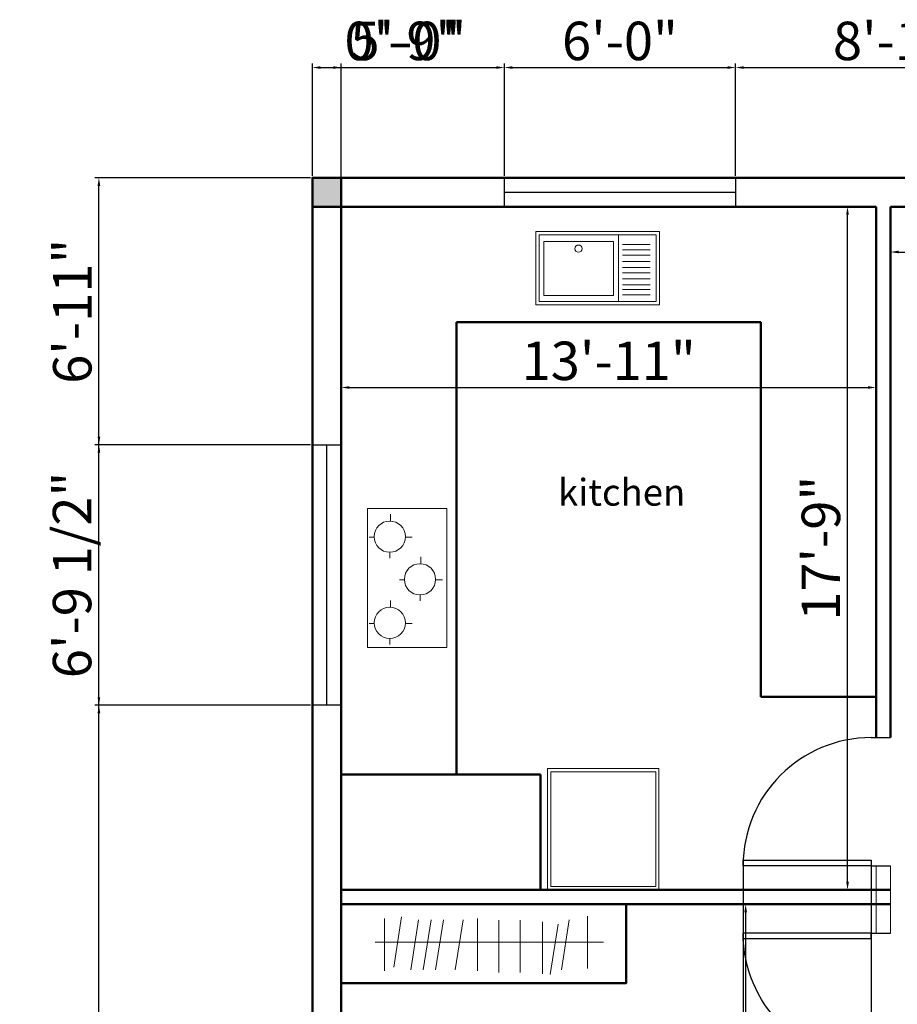
# Model space of a CAD drawing. Units: inches. Extents: x 1367 to 2309, y 1406 to 3826.
# Tile 2 of 9: x 1417 to 1691, y 1853 to 2160. Entities that reach past the tile are written whole.
import ezdxf

# ---------------------------------------------------------------- set-up
doc = ezdxf.new("R2010")
doc.units = ezdxf.units.IN
for name, color, linetype, lineweight in [('A-ANNO-DIMS', 2, 'Continuous', 18), ('A-AREA-IDEN', 3, 'Continuous', 18), ('A-DOOR', 4, 'Continuous', 25), ('A-FLOR-FIXT', 8, 'Continuous', 18), ('A-FURN', 8, 'Continuous', 18), ('A-GLAZ', 4, 'Continuous', 25), ('A-WALL', 7, 'Continuous', 50), ('A-WALL-PATT', 8, 'Continuous', 18)]:
    doc.layers.add(name, color=color, linetype=linetype, lineweight=lineweight)
doc.styles.get("Standard").update_dxf_attribs({"font": 'arial.ttf'})
doc.dimstyles.new('ISO-25', dxfattribs={"dimtxt": 12, "dimasz": 2.5, "dimexe": 1.25, "dimexo": 0.625, "dimtad": 1, "dimdec": 0, "dimlunit": 4, "dimtxsty": 'Standard', "dimcen": 2.5, "dimadec": 0, "dimazin": 0, "dimtfac": 1, "dimtdec": 0, "dimtmove": 0, "dimatfit": 3, "dimfxl": 1, "dimarcsym": 0})

# ---------------------------------------------------------------- blocks, each defined once
blk = doc.blocks.new('*U2')
for p, q in [((0, 0), (0, -6)), ((40, 0), (40, -6))]:
    blk.add_line(p, q)
blk.add_lwpolyline([(0, 0), (0, 40), (1.75, 40), (1.75, 0)], close=True)
blk.add_arc((0, 0), 40, 0, 90)
blk = doc.blocks.new('*D23')
at = {"layer": 'A-ANNO-DIMS', "color": 0, "lineweight": -2, "transparency": 16777216}
for p, q in [((1517.49, 2101.5), (1517.49, 2044.48)), ((1684.37, 2101.5), (1684.37, 2044.48)), ((1519.99, 2045.73), (1681.87, 2045.73))]:
    blk.add_line(p, q, dxfattribs=at)
at = {"layer": 'A-ANNO-DIMS', "color": 0, "lineweight": 100, "transparency": 16777216}
for points in [[(1519.99, 2046.15), (1519.99, 2045.32), (1517.49, 2045.73)], [(1681.87, 2046.15), (1681.87, 2045.32), (1684.37, 2045.73)]]:
    blk.add_solid(points, dxfattribs=at)
at = {"layer": 'Defpoints', "color": 0, "lineweight": 100, "transparency": 16777216}
for p in [(1517.49, 2102.13), (1684.37, 2102.13), (1684.37, 2045.73)]:
    blk.add_point(p, dxfattribs=at)
at = {"layer": 'A-ANNO-DIMS', "color": 0, "transparency": 16777216, "insert": (1600.93, 2052.49), "char_height": 12, "attachment_point": 5}
blk.add_mtext('13\'-11"', dxfattribs=at)
blk = doc.blocks.new('*D24')
at = {"layer": 'A-ANNO-DIMS', "color": 0, "lineweight": -2, "transparency": 16777216}
for p, q in [((1683.74, 2102.13), (1674.21, 2102.13)), ((1675.46, 1891.56), (1675.46, 2099.63)), ((1683.74, 1889.06), (1674.21, 1889.06))]:
    blk.add_line(p, q, dxfattribs=at)
at = {"layer": 'A-ANNO-DIMS', "color": 0, "lineweight": 100, "transparency": 16777216}
for points in [[(1675.04, 2099.63), (1675.88, 2099.63), (1675.46, 2102.13)], [(1675.04, 1891.56), (1675.88, 1891.56), (1675.46, 1889.06)]]:
    blk.add_solid(points, dxfattribs=at)
at = {"layer": 'Defpoints', "color": 0, "lineweight": 100, "transparency": 16777216}
for p in [(1675.46, 2102.13), (1684.37, 2102.13), (1684.37, 1889.06)]:
    blk.add_point(p, dxfattribs=at)
at = {"layer": 'A-ANNO-DIMS', "color": 0, "transparency": 16777216, "insert": (1668.71, 1995.59), "char_height": 12, "attachment_point": 5, "rotation": 90}
blk.add_mtext('17\'-9"', dxfattribs=at)
blk = doc.blocks.new('*D26')
at = {"layer": 'A-ANNO-DIMS', "color": 0, "lineweight": -2, "transparency": 16777216}
for p, q in [((1683.74, 1884.56), (1642.43, 1884.56)), ((1643.68, 1642.63), (1643.68, 1882.06)), ((1683.74, 1640.13), (1642.43, 1640.13))]:
    blk.add_line(p, q, dxfattribs=at)
at = {"layer": 'A-ANNO-DIMS', "color": 0, "lineweight": 100, "transparency": 16777216}
for points in [[(1643.26, 1882.06), (1644.09, 1882.06), (1643.68, 1884.56)], [(1643.26, 1642.63), (1644.09, 1642.63), (1643.68, 1640.13)]]:
    blk.add_solid(points, dxfattribs=at)
at = {"layer": 'Defpoints', "color": 0, "lineweight": 100, "transparency": 16777216}
for p in [(1643.68, 1884.56), (1684.37, 1884.56), (1684.37, 1640.13)]:
    blk.add_point(p, dxfattribs=at)
at = {"layer": 'A-ANNO-DIMS', "color": 0, "transparency": 16777216, "insert": (1636.93, 1762.34), "char_height": 12, "attachment_point": 5, "rotation": 90}
blk.add_mtext('20\'-4"', dxfattribs=at)
blk = doc.blocks.new('*D27')
at = {"layer": 'A-ANNO-DIMS', "color": 0, "lineweight": -2, "transparency": 16777216}
for p, q in [((1688.87, 2101.5), (1688.87, 2086.74)), ((1773.66, 2101.5), (1773.66, 2086.74)), ((1691.37, 2087.99), (1771.16, 2087.99))]:
    blk.add_line(p, q, dxfattribs=at)
at = {"layer": 'A-ANNO-DIMS', "color": 0, "lineweight": 100, "transparency": 16777216}
for points in [[(1691.37, 2088.41), (1691.37, 2087.58), (1688.87, 2087.99)], [(1771.16, 2088.41), (1771.16, 2087.58), (1773.66, 2087.99)]]:
    blk.add_solid(points, dxfattribs=at)
at = {"layer": 'Defpoints', "color": 0, "lineweight": 100, "transparency": 16777216}
for p in [(1688.87, 2102.13), (1773.66, 2102.13), (1773.66, 2087.99)]:
    blk.add_point(p, dxfattribs=at)
at = {"layer": 'A-ANNO-DIMS', "color": 0, "transparency": 16777216, "insert": (1731.27, 2094.64), "char_height": 12, "attachment_point": 5}
blk.add_mtext('7\'-1"', dxfattribs=at)
blk = doc.blocks.new('BURNER')
blk.add_line((9.74, 4.72), (11.92, 4.72))
blk.add_circle((4.87, 4.87), 4.87)
blk = doc.blocks.new('*D57')
at = {"layer": 'A-ANNO-DIMS', "color": 0, "lineweight": -2, "transparency": 16777216}
for p, q in [((1508.49, 2111.75), (1508.49, 2146.78)), ((1510.99, 2145.53), (1514.99, 2145.53)), ((1517.49, 2102.75), (1517.49, 2146.78)), ((1517.49, 2145.53), (1553.14, 2145.53))]:
    blk.add_line(p, q, dxfattribs=at)
at = {"layer": 'A-ANNO-DIMS', "color": 0, "lineweight": 100, "transparency": 16777216}
for points in [[(1510.99, 2145.94), (1510.99, 2145.11), (1508.49, 2145.53)], [(1514.99, 2145.94), (1514.99, 2145.11), (1517.49, 2145.53)]]:
    blk.add_solid(points, dxfattribs=at)
at = {"layer": 'Defpoints', "color": 0, "lineweight": 100, "transparency": 16777216}
for p in [(1517.49, 2145.53), (1508.49, 2111.13), (1517.49, 2102.13)]:
    blk.add_point(p, dxfattribs=at)
at = {"layer": 'A-ANNO-DIMS', "color": 0, "transparency": 16777216, "insert": (1536.57, 2152.28), "char_height": 12, "attachment_point": 5}
blk.add_mtext('0\'-9"', dxfattribs=at)
blk = doc.blocks.new('*D58')
at = {"layer": 'A-ANNO-DIMS', "color": 0, "lineweight": -2, "transparency": 16777216}
for p, q in [((1508.49, 2111.75), (1508.49, 2146.78)), ((1510.99, 2145.53), (1565.87, 2145.53)), ((1568.37, 2111.75), (1568.37, 2146.78))]:
    blk.add_line(p, q, dxfattribs=at)
at = {"layer": 'A-ANNO-DIMS', "color": 0, "lineweight": 100, "transparency": 16777216}
for points in [[(1510.99, 2145.94), (1510.99, 2145.11), (1508.49, 2145.53)], [(1565.87, 2145.94), (1565.87, 2145.11), (1568.37, 2145.53)]]:
    blk.add_solid(points, dxfattribs=at)
at = {"layer": 'Defpoints', "color": 0, "lineweight": 100, "transparency": 16777216}
for p in [(1568.37, 2145.53), (1508.49, 2111.13), (1568.37, 2111.13)]:
    blk.add_point(p, dxfattribs=at)
at = {"layer": 'A-ANNO-DIMS', "color": 0, "transparency": 16777216, "insert": (1538.43, 2152.28), "char_height": 12, "attachment_point": 5}
blk.add_mtext('5\'-0"', dxfattribs=at)
blk = doc.blocks.new('*D59')
at = {"layer": 'A-ANNO-DIMS', "color": 0, "lineweight": -2, "transparency": 16777216}
for p, q in [((1568.37, 2111.75), (1568.37, 2146.78)), ((1570.87, 2145.53), (1638.03, 2145.53)), ((1640.53, 2111.75), (1640.53, 2146.78))]:
    blk.add_line(p, q, dxfattribs=at)
at = {"layer": 'A-ANNO-DIMS', "color": 0, "lineweight": 100, "transparency": 16777216}
for points in [[(1570.87, 2145.94), (1570.87, 2145.11), (1568.37, 2145.53)], [(1638.03, 2145.94), (1638.03, 2145.11), (1640.53, 2145.53)]]:
    blk.add_solid(points, dxfattribs=at)
at = {"layer": 'Defpoints', "color": 0, "lineweight": 100, "transparency": 16777216}
for p in [(1640.53, 2145.53), (1568.37, 2111.13), (1640.53, 2111.13)]:
    blk.add_point(p, dxfattribs=at)
at = {"layer": 'A-ANNO-DIMS', "color": 0, "transparency": 16777216, "insert": (1604.45, 2152.28), "char_height": 12, "attachment_point": 5}
blk.add_mtext('6\'-0"', dxfattribs=at)
blk = doc.blocks.new('*D60')
at = {"layer": 'A-ANNO-DIMS', "color": 0, "lineweight": -2, "transparency": 16777216}
for p, q in [((1640.53, 2111.75), (1640.53, 2146.78)), ((1643.03, 2145.53), (1734.96, 2145.53)), ((1737.46, 2111.75), (1737.46, 2146.78))]:
    blk.add_line(p, q, dxfattribs=at)
at = {"layer": 'A-ANNO-DIMS', "color": 0, "lineweight": 100, "transparency": 16777216}
for points in [[(1643.03, 2145.94), (1643.03, 2145.11), (1640.53, 2145.53)], [(1734.96, 2145.94), (1734.96, 2145.11), (1737.46, 2145.53)]]:
    blk.add_solid(points, dxfattribs=at)
at = {"layer": 'Defpoints', "color": 0, "lineweight": 100, "transparency": 16777216}
for p in [(1737.46, 2145.53), (1640.53, 2111.13), (1737.46, 2111.13)]:
    blk.add_point(p, dxfattribs=at)
at = {"layer": 'A-ANNO-DIMS', "color": 0, "transparency": 16777216, "insert": (1688.99, 2152.28), "char_height": 12, "attachment_point": 5}
blk.add_mtext('8\'-1"', dxfattribs=at)
blk = doc.blocks.new('*D70')
at = {"layer": 'A-ANNO-DIMS', "color": 0, "lineweight": -2, "transparency": 16777216}
for p, q in [((1507.87, 2111.13), (1440.62, 2111.13)), ((1441.87, 1491.44), (1441.87, 2108.63)), ((1507.87, 1488.94), (1440.62, 1488.94))]:
    blk.add_line(p, q, dxfattribs=at)
at = {"layer": 'A-ANNO-DIMS', "color": 0, "lineweight": 100, "transparency": 16777216}
for points in [[(1441.45, 2108.63), (1442.28, 2108.63), (1441.87, 2111.13)], [(1441.45, 1491.44), (1442.28, 1491.44), (1441.87, 1488.94)]]:
    blk.add_solid(points, dxfattribs=at)
at = {"layer": 'Defpoints', "color": 0, "lineweight": 100, "transparency": 16777216}
for p in [(1441.87, 2111.13), (1508.49, 2111.13), (1508.49, 1488.94)]:
    blk.add_point(p, dxfattribs=at)
at = {"layer": 'A-ANNO-DIMS', "color": 0, "transparency": 16777216, "insert": (1435.11, 1800.03), "char_height": 12, "attachment_point": 5, "rotation": 90}
blk.add_mtext('51\'-10"', dxfattribs=at)
blk = doc.blocks.new('*D72')
at = {"layer": 'A-ANNO-DIMS', "color": 0, "lineweight": -2, "transparency": 16777216}
for p, q in [((1507.87, 1946.63), (1440.62, 1946.63)), ((1441.87, 1633.63), (1441.87, 1944.13)), ((1507.87, 1631.13), (1440.62, 1631.13))]:
    blk.add_line(p, q, dxfattribs=at)
at = {"layer": 'A-ANNO-DIMS', "color": 0, "lineweight": 100, "transparency": 16777216}
for points in [[(1441.45, 1944.13), (1442.28, 1944.13), (1441.87, 1946.63)], [(1441.45, 1633.63), (1442.28, 1633.63), (1441.87, 1631.13)]]:
    blk.add_solid(points, dxfattribs=at)
at = {"layer": 'Defpoints', "color": 0, "lineweight": 100, "transparency": 16777216}
for p in [(1441.87, 1946.63), (1508.49, 1946.63), (1508.49, 1631.13)]:
    blk.add_point(p, dxfattribs=at)
at = {"layer": 'A-ANNO-DIMS', "color": 0, "transparency": 16777216, "insert": (1435.03, 1788.88), "char_height": 12, "attachment_point": 5, "rotation": 90}
blk.add_mtext('26\'-3 1/2"', dxfattribs=at)
blk = doc.blocks.new('*D73')
at = {"layer": 'A-ANNO-DIMS', "color": 0, "lineweight": -2, "transparency": 16777216}
for p, q in [((1507.87, 2027.88), (1440.62, 2027.88)), ((1441.87, 1949.13), (1441.87, 2025.38)), ((1507.87, 1946.63), (1440.62, 1946.63))]:
    blk.add_line(p, q, dxfattribs=at)
at = {"layer": 'A-ANNO-DIMS', "color": 0, "lineweight": 100, "transparency": 16777216}
for points in [[(1441.45, 2025.38), (1442.28, 2025.38), (1441.87, 2027.88)], [(1441.45, 1949.13), (1442.28, 1949.13), (1441.87, 1946.63)]]:
    blk.add_solid(points, dxfattribs=at)
at = {"layer": 'Defpoints', "color": 0, "lineweight": 100, "transparency": 16777216}
for p in [(1441.87, 2027.88), (1508.49, 2027.88), (1508.49, 1946.63)]:
    blk.add_point(p, dxfattribs=at)
at = {"layer": 'A-ANNO-DIMS', "color": 0, "transparency": 16777216, "insert": (1435.04, 1987.26), "char_height": 12, "attachment_point": 5, "rotation": 90}
blk.add_mtext('6\'-9 1/2"', dxfattribs=at)
blk = doc.blocks.new('*D74')
at = {"layer": 'A-ANNO-DIMS', "color": 0, "lineweight": -2, "transparency": 16777216}
for p, q in [((1507.87, 2111.13), (1440.62, 2111.13)), ((1441.87, 2030.38), (1441.87, 2108.63)), ((1507.87, 2027.88), (1440.62, 2027.88))]:
    blk.add_line(p, q, dxfattribs=at)
at = {"layer": 'A-ANNO-DIMS', "color": 0, "lineweight": 100, "transparency": 16777216}
for points in [[(1441.45, 2108.63), (1442.28, 2108.63), (1441.87, 2111.13)], [(1441.45, 2030.38), (1442.28, 2030.38), (1441.87, 2027.88)]]:
    blk.add_solid(points, dxfattribs=at)
at = {"layer": 'Defpoints', "color": 0, "lineweight": 100, "transparency": 16777216}
for p in [(1441.87, 2111.13), (1508.49, 2111.13), (1508.49, 2027.88)]:
    blk.add_point(p, dxfattribs=at)
at = {"layer": 'A-ANNO-DIMS', "color": 0, "transparency": 16777216, "insert": (1435.11, 2069.51), "char_height": 12, "attachment_point": 5, "rotation": 90}
blk.add_mtext('6\'-11"', dxfattribs=at)
blk = doc.blocks.new('*D136')
at = {"layer": 'A-ANNO-DIMS', "color": 0, "lineweight": -2, "transparency": 16777216}
for p, q in [((1642.87, 1897.66), (1642.87, 1415.33)), ((1682.87, 1897.66), (1682.87, 1415.33)), ((1645.37, 1416.58), (1680.37, 1416.58))]:
    blk.add_line(p, q, dxfattribs=at)
at = {"layer": 'A-ANNO-DIMS', "color": 0, "lineweight": 100, "transparency": 16777216}
for points in [[(1645.37, 1416.99), (1645.37, 1416.16), (1642.87, 1416.58)], [(1680.37, 1416.99), (1680.37, 1416.16), (1682.87, 1416.58)]]:
    blk.add_solid(points, dxfattribs=at)
at = {"layer": 'Defpoints', "color": 0, "lineweight": 100, "transparency": 16777216}
for p in [(1642.87, 1898.28), (1682.87, 1898.28), (1682.87, 1416.58)]:
    blk.add_point(p, dxfattribs=at)
at = {"layer": 'A-ANNO-DIMS', "color": 0, "transparency": 16777216, "insert": (1662.87, 1423.33), "char_height": 12, "attachment_point": 5}
blk.add_mtext('3\'-4"', dxfattribs=at)

msp = doc.modelspace()

# ---------------------------------------------------------------- hatches: boundary and pattern name
at = {"layer": 'A-WALL-PATT'}
h = msp.add_hatch(color=256, dxfattribs=at)
h.dxf.hatch_style = 1
h.paths.add_polyline_path([(1517.49, 2102.13), (1517.49, 2111.13), (1508.49, 2111.13), (1508.49, 2102.13)])
h = msp.add_hatch(color=256, dxfattribs=at)
h.dxf.hatch_style = 1
h.paths.add_polyline_path([(1508.49, 1631.13), (1517.49, 1631.13), (1517.49, 1640.13), (1508.49, 1640.13)])
h.paths.add_polyline_path([(1773.99, 1631.13), (1782.99, 1631.13), (1782.99, 1640.13), (1773.99, 1640.13)])
h.paths.add_polyline_path([(1959.99, 1631.13), (1959.99, 1640.13), (1950.99, 1640.13), (1950.99, 1631.13)])
h.paths.add_polyline_path([(2099.49, 1640.13), (2099.49, 1631.13), (2108.49, 1631.13), (2108.49, 1640.13)])
h.paths.add_polyline_path([(1706.06, 1795.81), (1771.22, 1795.81), (1771.22, 1813.02), (1706.06, 1813.02)], flags=9)
h.paths.add_polyline_path([(1573.51, 1725.43), (1623.74, 1725.43), (1623.74, 1742.65), (1573.51, 1742.65)], flags=9)
h.paths.add_polyline_path([(1582.26, 2004.3), (1623.41, 2004.3), (1623.41, 2021.52), (1582.26, 2021.52)], flags=9)
h.paths.add_polyline_path([(1992.39, 1973.53), (2042.62, 1973.53), (2042.62, 1990.75), (1992.39, 1990.75)], flags=9)
h.paths.add_polyline_path([(2015.09, 1737.31), (2065.32, 1737.31), (2065.32, 1754.53), (2015.09, 1754.53)], flags=9)
h.paths.add_polyline_path([(1827.45, 1770.85), (1884.81, 1770.85), (1884.81, 1788.06), (1827.45, 1788.06)], flags=9)

# ---------------------------------------------------------------- linework, layer by layer
at = {"layer": 'A-FURN'}
for p, q in [((1603.95, 2072.55), (1603.95, 2093.38)), ((1605.24, 2090.36), (1613.84, 2090.36)), ((1605.24, 2088.72), (1613.84, 2088.72)), ((1605.24, 2087.03), (1613.84, 2087.03)), ((1605.24, 2085.06), (1613.84, 2085.06)), ((1605.24, 2083.21), (1613.84, 2083.21)), ((1605.24, 2081.47), (1613.84, 2081.47)), ((1605.24, 2079.61), (1613.84, 2079.61)), ((1605.24, 2077.76), (1613.84, 2077.76)), ((1605.24, 2076.3), (1613.84, 2076.3)), ((1605.24, 2074.61), (1613.84, 2074.61)), ((1532.84, 2004.07), (1532.84, 2006.22)), ((1527.74, 1999.06), (1526.16, 1999.06)), ((1532.66, 1994.34), (1532.66, 1992.47)), ((1542.28, 1990.75), (1542.28, 1992.9)), ((1537.18, 1985.74), (1535.61, 1985.74)), ((1542.11, 1981.02), (1542.11, 1979.15)), ((1532.84, 1977.16), (1532.84, 1979.3)), ((1527.74, 1972.14), (1526.16, 1972.14)), ((1532.66, 1967.42), (1532.66, 1965.56)), ((1684.37, 1896.53), (1684.37, 1875.57)), ((1688.87, 1896.53), (1688.87, 1875.57)), ((1530.96, 1863.76), (1530.96, 1880.07)), ((1533.84, 1864.91), (1536.3, 1880.58)), ((1539.17, 1864.06), (1541.62, 1879.73)), ((1543.05, 1864.06), (1545.5, 1879.73)), ((1546.93, 1864.06), (1549.38, 1879.73)), ((1553.06, 1864.06), (1555.52, 1879.73)), ((1559.95, 1863.76), (1559.95, 1880.07)), ((1586.17, 1864.06), (1588.63, 1879.73)), ((1594.34, 1864.53), (1594.34, 1880.84)), ((1530.96, 1877.33), (1530.96, 1863.76)), ((1566.64, 1863.25), (1566.64, 1879.56)), ((1573.34, 1863.25), (1573.34, 1879.56)), ((1580.26, 1862.79), (1580.26, 1879.1)), ((1582.71, 1862.65), (1585.17, 1878.32)), ((1528.04, 1872.69), (1599.31, 1872.69))]:
    msp.add_line(p, q, dxfattribs=at)
msp.add_lwpolyline([(1508.49, 2102.13), (1508.49, 2111.13), (1517.49, 2111.13)], dxfattribs=at)
for points in [[(1578.23, 2071.55), (1616.74, 2071.55), (1616.74, 2094.38), (1578.23, 2094.38)], [(1579.23, 2072.55), (1615.74, 2072.55), (1615.74, 2093.38), (1579.23, 2093.38)], [(1580.66, 2091.3), (1602.42, 2091.3), (1602.42, 2074.39), (1580.66, 2074.39)], [(1525.63, 1964.65), (1550.45, 1964.65), (1550.45, 2008.02), (1525.63, 2008.02)], [(1581.82, 1889.06), (1616.63, 1889.06), (1616.63, 1926.89), (1581.82, 1926.89)], [(1582.85, 1890.09), (1615.6, 1890.09), (1615.6, 1925.86), (1582.85, 1925.86)]]:
    msp.add_lwpolyline(points, close=True, dxfattribs=at)
msp.add_circle((1591.51, 2089.05), 1.12, dxfattribs=at)
at = {"layer": 'A-GLAZ'}
for p, q in [((1568.37, 2106.63), (1640.53, 2106.63)), ((1512.99, 1946.63), (1512.99, 2027.88))]:
    msp.add_line(p, q, dxfattribs=at)
for points in [[(1568.37, 2111.13), (1640.53, 2111.13), (1640.53, 2102.13), (1568.37, 2102.13)], [(1508.49, 2027.88), (1517.49, 2027.88), (1517.49, 1946.63), (1508.49, 1946.63)]]:
    msp.add_lwpolyline(points, close=True, dxfattribs=at)
at = {"layer": 'A-WALL'}
for p, q in [((1517.49, 2102.13), (1684.37, 2102.13)), ((1517.49, 2102.13), (1517.49, 2066.13)), ((1684.37, 2102.13), (1684.37, 1936.53)), ((1688.87, 2102.13), (1688.87, 1936.53)), ((1688.87, 2102.13), (1746.15, 2102.13)), ((1553.49, 2066.13), (1648.37, 2066.13)), ((1553.49, 1925.06), (1553.49, 2066.13)), ((1648.37, 1949.23), (1648.37, 2066.13)), ((1660.37, 1949.23), (1648.37, 1949.23)), ((1684.37, 1949.23), (1660.37, 1949.23)), ((1517.49, 1889.06), (1517.49, 1925.06)), ((1517.49, 1925.06), (1579.67, 1925.06)), ((1579.67, 1925.06), (1579.67, 1889.06)), ((1517.49, 1889.06), (1688.87, 1889.06)), ((1517.49, 1889.06), (1553.49, 1889.06)), ((1517.49, 1884.56), (1688.87, 1884.56))]:
    msp.add_line(p, q, dxfattribs=at)
for points in [[(1751.28, 1631.13), (2108.49, 1631.13), (2108.49, 2111.13), (1508.49, 2111.13), (1508.49, 1631.13), (1711.28, 1631.13)], [(1684.37, 2102.13), (1517.49, 2102.13), (1517.49, 1804.12)], [(2099.49, 1808.62), (2099.49, 2102.13), (1688.87, 2102.13)]]:
    msp.add_lwpolyline(points, dxfattribs=at)
for points in [[(1517.49, 2102.13), (1508.49, 2102.13), (1508.49, 2111.13), (1517.49, 2111.13)], [(1517.49, 1884.56), (1517.49, 1859.92), (1606.35, 1859.92), (1606.35, 1884.56)]]:
    msp.add_lwpolyline(points, close=True, dxfattribs=at)

# ---------------------------------------------------------------- block references
at = {"layer": 'A-DOOR', "rotation": 90}
msp.add_blockref('*U2', (1682.87, 1896.53), dxfattribs=at)
at = {"layer": 'A-DOOR', "xscale": -1, "rotation": 90}
msp.add_blockref('*U2', (1682.87, 1875.57), dxfattribs=at)
at = {"layer": 'A-FLOR-FIXT'}
for p in [(1527.74, 1994.34), (1537.18, 1981.02), (1527.74, 1967.42)]:
    msp.add_blockref('BURNER', p, dxfattribs=at)

# ---------------------------------------------------------------- texts
at = {"layer": 'A-AREA-IDEN', "insert": (1585.12, 2017.22), "char_height": 8.353, "attachment_point": 1}
msp.add_mtext_dynamic_manual_height_columns('kitchen', width=204.251, gutter_width=41.76, heights=[0], dxfattribs=at)

# ---------------------------------------------------------------- dimensions: what is measured, and where the dimension line sits
at = {"layer": 'A-ANNO-DIMS'}
for base, p1, p2, override, picture, middle in [((1517.49, 2145.53), (1508.49, 2111.13), (1517.49, 2102.13), {"dimdec": 1, "dimlfac": 1, "dimrnd": 0, "dimzin": 1, "dimdsep": 46, "dimlunit": 4, "dimfrac": 2}, '*D57', (1536.57, 2152.28)), ((1568.37, 2145.53), (1508.49, 2111.13), (1568.37, 2111.13), {"dimdec": 1, "dimlfac": 1, "dimrnd": 0, "dimzin": 1, "dimdsep": 46, "dimlunit": 4, "dimfrac": 2}, '*D58', (1538.43, 2152.28)), ((1640.53, 2145.53), (1568.37, 2111.13), (1640.53, 2111.13), {"dimdec": 1, "dimlfac": 1, "dimrnd": 0, "dimzin": 1, "dimdsep": 46, "dimlunit": 4, "dimfrac": 2}, '*D59', (1604.45, 2152.28)), ((1737.46, 2145.53), (1640.53, 2111.13), (1737.46, 2111.13), {"dimdec": 1, "dimlfac": 1, "dimrnd": 0, "dimzin": 1, "dimdsep": 46, "dimlunit": 4, "dimfrac": 2}, '*D60', (1688.99, 2152.28)), ((1684.37, 2045.73), (1517.49, 2102.13), (1684.37, 2102.13), {"dimclrd": 0, "dimclre": 0, "dimclrt": 0}, '*D23', (1600.93, 2052.49)), ((1773.66, 2087.99), (1688.87, 2102.13), (1773.66, 2102.13), {"dimclrd": 0, "dimclre": 0, "dimclrt": 0}, '*D27', (1731.27, 2094.64)), ((1682.87, 1416.58), (1642.87, 1898.28), (1682.87, 1898.28), {"dimdec": 1, "dimlfac": 1, "dimrnd": 0, "dimzin": 1, "dimdsep": 46, "dimlunit": 4, "dimfrac": 2}, '*D136', (1662.87, 1423.33))]:
    dim = msp.add_linear_dim(base=base, p1=p1, p2=p2, dimstyle='ISO-25', override=override, dxfattribs=at)
    dim.commit()
    dim.dimension.update_dxf_attribs({"geometry": picture, "text_midpoint": middle})
for base, p1, p2, override, picture, middle in [((1441.87, 2111.13), (1508.49, 1488.94), (1508.49, 2111.13), {"dimdec": 1, "dimlfac": 1, "dimrnd": 0, "dimzin": 1, "dimdsep": 46, "dimlunit": 4, "dimfrac": 2}, '*D70', (1435.11, 1800.03)), ((1441.8656, 2111.128), (1508.4928, 2027.8841), (1508.4928, 2111.128), {"dimdec": 1, "dimlfac": 1, "dimrnd": 0, "dimzin": 1, "dimdsep": 46, "dimlunit": 4, "dimfrac": 2}, '*D74', (1435.1137, 2069.506)), ((1675.46, 2102.13), (1684.37, 1889.06), (1684.37, 2102.13), {"dimclrd": 0, "dimclre": 0, "dimclrt": 0}, '*D24', (1668.71, 1995.59)), ((1441.8656, 2027.8841), (1508.4928, 1946.632), (1508.4928, 2027.8841), {"dimdec": 1, "dimlfac": 1, "dimrnd": 0, "dimzin": 1, "dimdsep": 46, "dimlunit": 4, "dimfrac": 2}, '*D73', (1435.036, 1987.258)), ((1441.87, 1946.63), (1508.49, 1631.13), (1508.49, 1946.63), {"dimdec": 1, "dimlfac": 1, "dimrnd": 0, "dimzin": 1, "dimdsep": 46, "dimlunit": 4, "dimfrac": 2}, '*D72', (1435.03, 1788.88)), ((1643.68, 1884.56), (1684.37, 1640.13), (1684.37, 1884.56), {"dimclrd": 0, "dimclre": 0, "dimclrt": 0}, '*D26', (1636.93, 1762.34))]:
    dim = msp.add_linear_dim(base=base, p1=p1, p2=p2, angle=90, dimstyle='ISO-25', override=override, dxfattribs=at)
    dim.commit()
    dim.dimension.update_dxf_attribs({"geometry": picture, "text_midpoint": middle})

doc.saveas('drawing.dxf')
